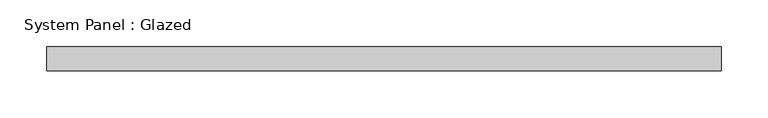
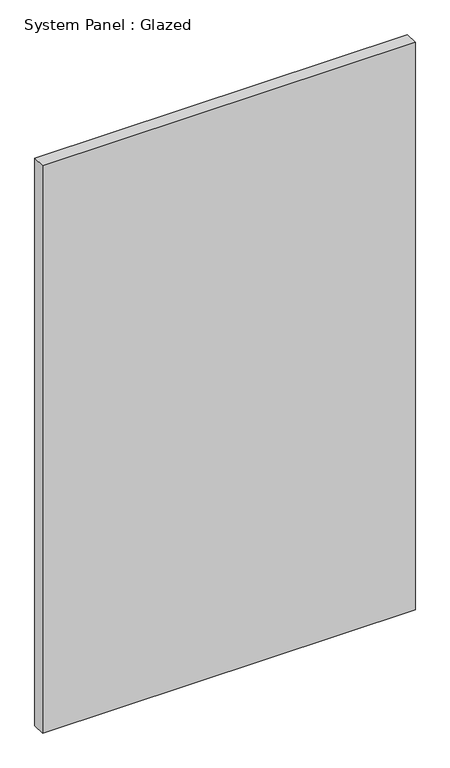
"""IFC4 building model written with IfcOpenShell, lengths in millimetres: plate geometry, System Panel : Glazed."""

from ifc_helpers import new_model, si_unit, origin, origin_with_axes, place, context, project, spatial, polyline, outline, extrude, source, transform, mapped, element, save


def system_panel_glazed_4f3cd66b(model_context):
    return source(origin(), model_context, "Body", "SweptSolid", [
        extrude(outline(polyline([(359.5150734, 19.05), (-359.5150734, 19.05), (-359.5150734, 44.45), (359.5150734, 44.45), (359.5150734, 19.05)])), origin_with_axes(), (0.0, 0.0, 1.0), 1155.7),
    ])


if __name__ == "__main__":
    model = new_model("IFC4")
    model_context = context("Model", 3, world=origin())
    ifc_project = project(units=[si_unit("LENGTHUNIT", "METRE", prefix="MILLI")], contexts=[model_context])
    site = spatial("IfcSite", under=ifc_project)
    building = spatial("IfcBuilding", under=site)
    placement = place(None, origin())
    system_panel_glazed_shape = system_panel_glazed_4f3cd66b(model_context)
    element("IfcPlate", 1, ObjectType="System Panel : Glazed", at=placement, inside=building, context=model_context, shape_type="MappedRepresentation", body=[
        mapped(system_panel_glazed_shape, transform((0.0, 0.0, 0.0), x_axis=(1.0, 0.0, 0.0), y_axis=(0.0, 1.0, 0.0), z_axis=(0.0, 0.0, 1.0))),
    ])
    save(model, "model.ifc")

# Revit data of these elements
# Type "System Panel : Glazed"
#   Construction Type Id = "GSP4R"
#   Analytic Construction = "1/8 in Pilkington single glazing"
#   Visual Light Transmittance = 0.9
#   Solar Heat Gain Coefficient = 0.86
#   Heat Transfer Coefficient (U) = 1.18115 BTU/(h·ft²·°F)
# Element 1 (IfcPlate, "System Panel : Glazed")
#   Materials on its faces: "Glass"
# Materials
#   "Glass": class "Glass", colour RGB 0 128 192, transparency 0.75, Description = "Soda Lime Glass", Cost = 0
